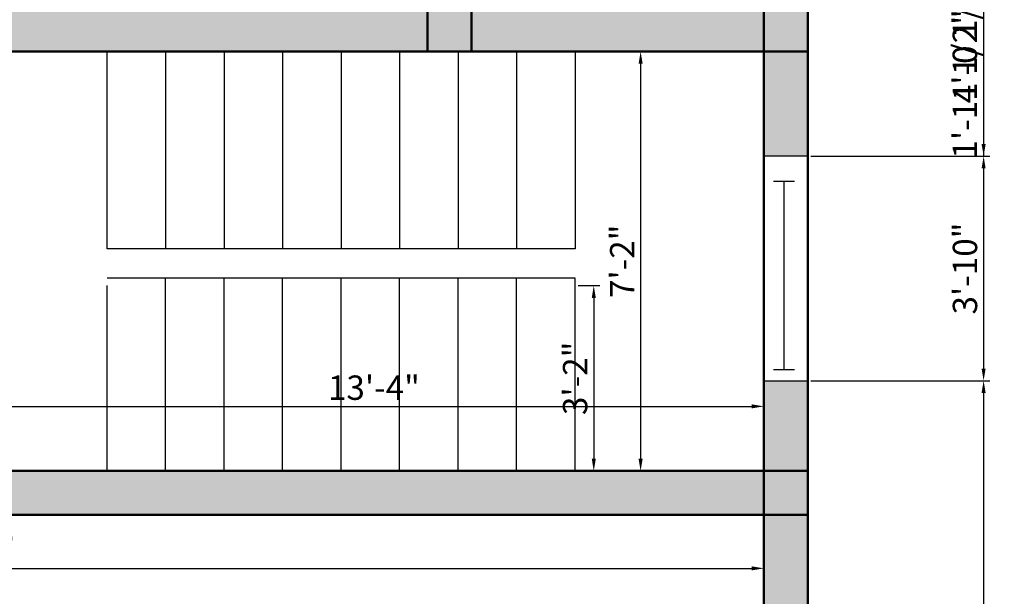
# Model space of a CAD drawing. Units: millimetres. Extents: x 2784 to 3697, y 603 to 1406.
# Tile 4 of 10: x 3013 to 3215, y 959 to 1077. Entities that reach past the tile are written whole.
import ezdxf

# ---------------------------------------------------------------- set-up
doc = ezdxf.new("R2010")
doc.units = ezdxf.units.MM
for name, color, linetype, lineweight in [('A-ANNO-DIMS', 140, 'Continuous', 18), ('A-FLOR-STRS', 200, 'Continuous', 25), ('A-GLAZ', 30, 'Continuous', 25), ('A-WALL', 2, 'Continuous', 50), ('A-WALL-PATT', 8, 'Continuous', 13)]:
    doc.layers.add(name, color=color, linetype=linetype, lineweight=lineweight)
doc.styles.get("Standard").update_dxf_attribs({"font": 'arial.ttf'})
doc.dimstyles.new('ISO-25', dxfattribs={"dimtxt": 5, "dimasz": 2.5, "dimexe": 1.25, "dimexo": 0.625, "dimtad": 1, "dimdec": 0, "dimlunit": 3, "dimtxsty": 'Standard', "dimcen": 2.5, "dimadec": 0, "dimazin": 0, "dimtfac": 1, "dimtdec": 0, "dimtmove": 0, "dimatfit": 3, "dimfxl": 1, "dimarcsym": 0})

# ---------------------------------------------------------------- blocks, each defined once
blk = doc.blocks.new('*U4')
for p, q in [((0, 4), (0, 0)), ((36, 4), (36, 0)), ((0, 2), (36, 2))]:
    blk.add_line(p, q)
blk = doc.blocks.new('*D27')
at = {"layer": 'A-ANNO-DIMS', "color": 0, "lineweight": -2, "transparency": 16777216}
for p, q in [((3005.91, 1000.77), (3005.91, 996.23)), ((3165.91, 1000.77), (3165.91, 996.23)), ((3008.41, 997.48), (3163.41, 997.48))]:
    blk.add_line(p, q, dxfattribs=at)
at = {"layer": 'A-ANNO-DIMS', "color": 0, "transparency": 16777216}
for points in [[(3008.41, 997.9), (3008.41, 997.06), (3005.91, 997.48)], [(3163.41, 997.9), (3163.41, 997.06), (3165.91, 997.48)]]:
    blk.add_solid(points, dxfattribs=at)
at = {"layer": 'Defpoints', "color": 0, "transparency": 16777216}
for p in [(3005.91, 1001.39), (3165.91, 1001.39), (3165.91, 997.48)]:
    blk.add_point(p, dxfattribs=at)
at = {"layer": 'A-ANNO-DIMS', "color": 0, "transparency": 16777216, "insert": (3085.91, 1000.66), "char_height": 5, "attachment_point": 5}
blk.add_mtext('13\'-4"', dxfattribs=at)
blk = doc.blocks.new('*D28')
at = {"layer": 'A-ANNO-DIMS', "color": 0, "lineweight": -2, "transparency": 16777216}
for p, q in [((3141.26, 1070.23), (3141.88, 1070.23)), ((3140.63, 1067.73), (3140.63, 986.73)), ((3141.26, 984.23), (3141.88, 984.23))]:
    blk.add_line(p, q, dxfattribs=at)
at = {"layer": 'A-ANNO-DIMS', "color": 0, "transparency": 16777216}
for points in [[(3140.21, 1067.73), (3141.05, 1067.73), (3140.63, 1070.23)], [(3140.21, 986.73), (3141.05, 986.73), (3140.63, 984.23)]]:
    blk.add_solid(points, dxfattribs=at)
at = {"layer": 'Defpoints', "color": 0, "transparency": 16777216}
for p in [(3140.63, 1070.23), (3140.63, 984.23), (3140.63, 984.23)]:
    blk.add_point(p, dxfattribs=at)
at = {"layer": 'A-ANNO-DIMS', "color": 0, "transparency": 16777216, "insert": (3137.5, 1027.23), "char_height": 5, "attachment_point": 5, "rotation": 90}
blk.add_mtext('7\'-2"', dxfattribs=at)
blk = doc.blocks.new('*D29')
at = {"layer": 'A-ANNO-DIMS', "color": 0, "lineweight": -2, "transparency": 16777216}
for p, q in [((3127.81, 1022.23), (3132.27, 1022.23)), ((3131.02, 1019.73), (3131.02, 986.73)), ((3127.81, 984.23), (3132.27, 984.23))]:
    blk.add_line(p, q, dxfattribs=at)
at = {"layer": 'A-ANNO-DIMS', "color": 0, "transparency": 16777216}
for points in [[(3130.61, 1019.73), (3131.44, 1019.73), (3131.02, 1022.23)], [(3130.61, 986.73), (3131.44, 986.73), (3131.02, 984.23)]]:
    blk.add_solid(points, dxfattribs=at)
at = {"layer": 'Defpoints', "color": 0, "transparency": 16777216}
for p in [(3127.18, 1022.23), (3127.18, 984.23), (3131.02, 984.23)]:
    blk.add_point(p, dxfattribs=at)
at = {"layer": 'A-ANNO-DIMS', "color": 0, "transparency": 16777216, "insert": (3127.84, 1003.23), "char_height": 5, "attachment_point": 5, "rotation": 90}
blk.add_mtext('3\'-2"', dxfattribs=at)
blk = doc.blocks.new('*D35')
at = {"layer": 'A-ANNO-DIMS', "color": 0, "lineweight": -2, "transparency": 16777216}
for p, q in [((2839.91, 959.54), (2839.91, 965.51)), ((2842.41, 964.26), (3163.41, 964.26)), ((3165.91, 959.54), (3165.91, 965.51))]:
    blk.add_line(p, q, dxfattribs=at)
at = {"layer": 'A-ANNO-DIMS', "color": 0, "transparency": 16777216}
for points in [[(2842.41, 964.68), (2842.41, 963.84), (2839.91, 964.26)], [(3163.41, 964.68), (3163.41, 963.84), (3165.91, 964.26)]]:
    blk.add_solid(points, dxfattribs=at)
at = {"layer": 'Defpoints', "color": 0, "transparency": 16777216}
for p in [(3165.91, 964.26), (2839.91, 958.92), (3165.91, 958.92)]:
    blk.add_point(p, dxfattribs=at)
at = {"layer": 'A-ANNO-DIMS', "color": 0, "transparency": 16777216, "insert": (3002.91, 967.39), "char_height": 5, "attachment_point": 5}
blk.add_mtext('27\'-2"', dxfattribs=at)
blk = doc.blocks.new('*D97')
at = {"layer": 'A-ANNO-DIMS', "color": 0, "lineweight": -2, "transparency": 16777216}
for p, q in [((3175.53, 1097.37), (3212.26, 1097.37)), ((3211.01, 1094.87), (3211.01, 1051.27)), ((3175.53, 1048.77), (3212.26, 1048.77))]:
    blk.add_line(p, q, dxfattribs=at)
at = {"layer": 'A-ANNO-DIMS', "color": 0, "transparency": 16777216}
for points in [[(3210.59, 1094.87), (3211.42, 1094.87), (3211.01, 1097.37)], [(3210.59, 1051.27), (3211.42, 1051.27), (3211.01, 1048.77)]]:
    blk.add_solid(points, dxfattribs=at)
at = {"layer": 'Defpoints', "color": 0, "transparency": 16777216}
for p in [(3174.91, 1097.37), (3174.91, 1048.77), (3211.01, 1048.77)]:
    blk.add_point(p, dxfattribs=at)
at = {"layer": 'A-ANNO-DIMS', "color": 0, "transparency": 16777216, "insert": (3207.8, 1073.07), "char_height": 5, "attachment_point": 5, "rotation": 90}
blk.add_mtext('4\'-0 1/2"', dxfattribs=at)
blk = doc.blocks.new('*D98')
at = {"layer": 'A-ANNO-DIMS', "color": 0, "lineweight": -2, "transparency": 16777216}
for p, q in [((3175.53, 1048.77), (3212.26, 1048.77)), ((3211.01, 1046.27), (3211.01, 1005.24)), ((3175.53, 1002.74), (3212.26, 1002.74))]:
    blk.add_line(p, q, dxfattribs=at)
at = {"layer": 'A-ANNO-DIMS', "color": 0, "transparency": 16777216}
for points in [[(3210.59, 1046.27), (3211.42, 1046.27), (3211.01, 1048.77)], [(3210.59, 1005.24), (3211.42, 1005.24), (3211.01, 1002.74)]]:
    blk.add_solid(points, dxfattribs=at)
at = {"layer": 'Defpoints', "color": 0, "transparency": 16777216}
for p in [(3174.91, 1048.77), (3174.91, 1002.74), (3211.01, 1002.74)]:
    blk.add_point(p, dxfattribs=at)
at = {"layer": 'A-ANNO-DIMS', "color": 0, "transparency": 16777216, "insert": (3207.83, 1025.75), "char_height": 5, "attachment_point": 5, "rotation": 90}
blk.add_mtext('3\'-10"', dxfattribs=at)
blk = doc.blocks.new('*D99')
at = {"layer": 'A-ANNO-DIMS', "color": 0, "lineweight": -2, "transparency": 16777216}
for p, q in [((3175.53, 1002.74), (3212.26, 1002.74)), ((3211.01, 1000.24), (3211.01, 646.1)), ((3175.53, 643.6), (3212.26, 643.6))]:
    blk.add_line(p, q, dxfattribs=at)
at = {"layer": 'A-ANNO-DIMS', "color": 0, "transparency": 16777216}
for points in [[(3210.59, 1000.24), (3211.42, 1000.24), (3211.01, 1002.74)], [(3210.59, 646.1), (3211.42, 646.1), (3211.01, 643.6)]]:
    blk.add_solid(points, dxfattribs=at)
at = {"layer": 'Defpoints', "color": 0, "transparency": 16777216}
for p in [(3174.91, 1002.74), (3174.91, 643.6), (3211.01, 643.6)]:
    blk.add_point(p, dxfattribs=at)
at = {"layer": 'A-ANNO-DIMS', "color": 0, "transparency": 16777216, "insert": (3207.83, 823.17), "char_height": 5, "attachment_point": 5, "rotation": 90}
blk.add_mtext('29\'-11"', dxfattribs=at)
blk = doc.blocks.new('*D107')
at = {"layer": 'A-ANNO-DIMS', "color": 0, "lineweight": -2, "transparency": 16777216}
for p, q in [((3105.04, 1104.19), (3212.26, 1104.19)), ((3211.01, 1101.69), (3211.01, 1083.41)), ((3106.53, 1080.91), (3212.26, 1080.91)), ((3211.01, 1080.91), (3211.01, 1048.8))]:
    blk.add_line(p, q, dxfattribs=at)
at = {"layer": 'A-ANNO-DIMS', "color": 0, "transparency": 16777216}
for points in [[(3210.59, 1101.69), (3211.42, 1101.69), (3211.01, 1104.19)], [(3210.59, 1083.41), (3211.42, 1083.41), (3211.01, 1080.91)]]:
    blk.add_solid(points, dxfattribs=at)
at = {"layer": 'Defpoints', "color": 0, "transparency": 16777216}
for p in [(3104.41, 1104.19), (3105.91, 1080.91), (3211.01, 1080.91)]:
    blk.add_point(p, dxfattribs=at)
at = {"layer": 'A-ANNO-DIMS', "color": 0, "transparency": 16777216, "insert": (3207.8, 1063.61), "char_height": 5, "attachment_point": 5, "rotation": 90}
blk.add_mtext('1\'-11 1/2"', dxfattribs=at)

msp = doc.modelspace()

# ---------------------------------------------------------------- hatches: boundary and pattern name
at = {"layer": 'A-WALL-PATT'}
h = msp.add_hatch(color=256, dxfattribs=at)
h.dxf.hatch_style = 1
h.paths.add_polyline_path([(2869.53, 1356.23), (2839.91, 1356.23), (2839.91, 1347.23), (2869.53, 1347.23)])
h.paths.add_polyline_path([(2839.91, 1356.23), (2830.91, 1356.23), (2830.91, 1347.23), (2839.91, 1347.23)])
h.paths.add_polyline_path([(2839.91, 1347.23), (2830.91, 1347.23), (2830.91, 1314.23), (2839.91, 1314.23)])
h.paths.add_polyline_path([(2839.91, 1268.19), (2830.91, 1268.19), (2830.91, 1222.23), (2839.91, 1222.23)])
h.paths.add_polyline_path([(2839.91, 1222.23), (2830.91, 1222.23), (2830.91, 1213.23), (2839.91, 1213.23)])
h.paths.add_polyline_path([(2962.91, 1222.23), (2839.91, 1222.23), (2839.91, 1213.23), (2962.91, 1213.23)])
h.paths.add_polyline_path([(2971.91, 1222.23), (2962.91, 1222.23), (2962.91, 1213.23), (2971.91, 1213.23)])
h.paths.add_polyline_path([(2971.91, 1263.23), (2962.91, 1263.23), (2962.91, 1254.23), (2971.91, 1254.23)])
h.paths.add_polyline_path([(2971.91, 1347.23), (2962.91, 1347.23), (2962.91, 1263.23), (2971.91, 1263.23)])
h.paths.add_polyline_path([(2971.91, 1356.23), (2962.91, 1356.23), (2962.91, 1347.23), (2971.91, 1347.23)])
h.paths.add_polyline_path([(2962.91, 1356.23), (2913.7, 1356.23), (2913.7, 1347.23), (2962.91, 1347.23)])
h.paths.add_polyline_path([(2982.62, 1356.23), (2971.91, 1356.23), (2971.91, 1347.23), (2982.62, 1347.23)])
h.paths.add_polyline_path([(3019.91, 1356.23), (3004.44, 1356.23), (3004.44, 1347.23), (3019.91, 1347.23)])
h.paths.add_polyline_path([(3028.91, 1356.23), (3019.91, 1356.23), (3019.91, 1347.23), (3028.91, 1347.23)])
h.paths.add_polyline_path([(3028.91, 1347.23), (3019.91, 1347.23), (3019.91, 1287.35, -0.06506), (3026.12, 1288.16), (3028.91, 1288.16)])
h.paths.add_polyline_path([(3019.91, 1263.23), (2971.91, 1263.23), (2971.91, 1254.23), (3019.91, 1254.23)])
h.paths.add_polyline_path([(3028.91, 1263.23), (3019.91, 1263.23), (3019.91, 1254.23), (3028.91, 1254.23)])
h.paths.add_polyline_path([(3028.91, 1254.23), (3019.91, 1254.23), (3019.91, 1222.23), (3028.91, 1222.23)])
h.paths.add_polyline_path([(3028.91, 1222.23), (3019.91, 1222.23), (3019.91, 1213.23), (3028.91, 1213.23)])
h.paths.add_polyline_path([(3165.91, 1222.23), (3060.65, 1222.23, -0.056956), (3061.45, 1215.23), (3061.45, 1213.23), (3165.91, 1213.23)])
h.paths.add_polyline_path([(3080.34, 1356.23), (3028.91, 1356.23), (3028.91, 1347.23), (3080.34, 1347.23)])
h.paths.add_polyline_path([(3174.91, 1347.23), (3165.91, 1347.23), (3165.91, 1311.28), (3174.91, 1311.28)])
h.paths.add_polyline_path([(3174.91, 1356.23), (3165.91, 1356.23), (3165.91, 1347.23), (3174.91, 1347.23)])
h.paths.add_polyline_path([(3165.91, 1356.23), (3123.1, 1356.23), (3123.1, 1347.23), (3165.91, 1347.23)])
h.paths.add_polyline_path([(3174.91, 1266.65), (3165.91, 1266.65), (3165.91, 1222.23), (3174.91, 1222.23)])
h.paths.add_polyline_path([(3174.91, 1222.23), (3165.91, 1222.23), (3165.91, 1213.23), (3174.91, 1213.23)])
h.paths.add_polyline_path([(3174.91, 1213.23), (3165.91, 1213.23), (3165.91, 1194.83), (3174.91, 1194.83)])
h.paths.add_polyline_path([(3105.91, 1182.92, -0.096276), (3096.91, 1180.92), (3096.91, 1148.23), (3105.91, 1148.23)])
h.paths.add_polyline_path([(3105.91, 1213.23), (3096.91, 1213.23), (3096.91, 1205.07), (3105.91, 1205.07)])
h.paths.add_polyline_path([(2971.91, 1213.23), (2962.91, 1213.23), (2962.91, 1161.09), (2971.91, 1161.09)])
h.paths.add_polyline_path([(2839.91, 1213.23), (2830.91, 1213.23), (2830.91, 1157.46), (2839.91, 1157.46)])
h.paths.add_polyline_path([(2839.91, 1108.88), (2830.91, 1108.88), (2830.91, 1042.23), (2839.91, 1042.23)])
h.paths.add_polyline_path([(2839.91, 1042.23), (2830.91, 1042.23), (2830.91, 1033.23), (2839.91, 1033.23)])
h.paths.add_polyline_path([(2881.91, 1042.23), (2839.91, 1042.23), (2839.91, 1033.23), (2881.91, 1033.23)])
h.paths.add_polyline_path([(2996.91, 1042.23), (2890.91, 1042.23), (2890.91, 1033.23), (2996.91, 1033.23)])
h.paths.add_polyline_path([(2890.91, 1042.23), (2881.91, 1042.23), (2881.91, 1033.23), (2890.91, 1033.23)])
h.paths.add_polyline_path([(2890.91, 1033.23), (2881.91, 1033.23), (2881.91, 984.23), (2890.91, 984.23)])
h.paths.add_polyline_path([(2839.91, 1033.23), (2830.91, 1033.23), (2830.91, 984.23), (2839.91, 984.23)])
h.paths.add_polyline_path([(2839.91, 984.23), (2830.91, 984.23), (2830.91, 975.23), (2839.91, 975.23)])
h.paths.add_polyline_path([(2881.91, 984.23), (2854.14, 984.23, -0.154991), (2857.05, 975.23), (2881.91, 975.23)])
h.paths.add_polyline_path([(2890.91, 984.23), (2881.91, 984.23), (2881.91, 975.23), (2890.91, 975.23)])
h.paths.add_polyline_path([(2900.85, 984.23), (2890.91, 984.23), (2890.91, 975.23), (2900.85, 975.23), (2900.85, 975.78)])
h.paths.add_polyline_path([(2996.91, 984.23), (2923.49, 984.23, -0.089525), (2925.01, 975.78), (2925.01, 975.23), (2996.91, 975.23)])
h.paths.add_polyline_path([(3165.91, 984.23), (3005.91, 984.23), (3005.91, 975.23), (3165.91, 975.23)])
h.paths.add_polyline_path([(3005.91, 1033.23), (2996.91, 1033.23), (2996.91, 984.23), (3005.91, 984.23)])
h.paths.add_polyline_path([(3005.91, 984.23), (2996.91, 984.23), (2996.91, 975.23), (3005.91, 975.23)])
h.paths.add_polyline_path([(3005.91, 1042.23), (2996.91, 1042.23), (2996.91, 1033.23), (3005.91, 1033.23)])
h.paths.add_polyline_path([(3096.91, 1079.23), (2971.91, 1079.23), (2971.91, 1070.23), (3096.91, 1070.23)])
h.paths.add_polyline_path([(2971.91, 1079.23), (2962.91, 1079.23), (2962.91, 1070.23), (2971.91, 1070.23)])
h.paths.add_polyline_path([(2971.91, 1070.23), (2962.91, 1070.23), (2962.91, 1060.28, -0.115005), (2971.91, 1066.55)])
h.paths.add_polyline_path([(2971.91, 1105.54), (2962.91, 1105.54), (2962.91, 1079.23), (2971.91, 1079.23)])
h.paths.add_polyline_path([(3165.91, 1079.23), (3105.91, 1079.23), (3105.91, 1070.23), (3165.91, 1070.23)])
h.paths.add_polyline_path([(3105.91, 1079.23), (3096.91, 1079.23), (3096.91, 1070.23), (3105.91, 1070.23)])
h.paths.add_polyline_path([(3105.91, 1148.23), (3096.91, 1148.23), (3096.91, 1139.23), (3105.91, 1139.23)])
h.paths.add_polyline_path([(3105.91, 1139.23), (3096.91, 1139.23), (3096.91, 1104.7), (3098.08, 1104.75, -0.08216), (3105.91, 1103.81)])
h.paths.add_polyline_path([(3165.91, 1148.23), (3105.91, 1148.23), (3105.91, 1139.23), (3165.91, 1139.23)])
h.paths.add_polyline_path([(3174.91, 1148.23), (3165.91, 1148.23), (3165.91, 1139.23), (3174.91, 1139.23)])
h.paths.add_polyline_path([(3174.91, 1139.23), (3165.91, 1139.23), (3165.91, 1123.86), (3174.91, 1123.86)])
h.paths.add_polyline_path([(3174.91, 1097.37), (3165.91, 1097.37), (3165.91, 1079.23), (3174.91, 1079.23)])
h.paths.add_polyline_path([(3174.91, 1079.23), (3165.91, 1079.23), (3165.91, 1070.23), (3174.91, 1070.23)])
h.paths.add_polyline_path([(3174.91, 1070.23), (3165.91, 1070.23), (3165.91, 1048.77), (3174.91, 1048.77)])
h.paths.add_polyline_path([(3174.91, 1002.74), (3165.91, 1002.74), (3165.91, 984.23), (3174.91, 984.23)])
h.paths.add_polyline_path([(3174.91, 984.23), (3165.91, 984.23), (3165.91, 975.23), (3174.91, 975.23)])
h.paths.add_polyline_path([(3174.91, 975.23), (3165.91, 975.23), (3165.91, 725.23), (3174.91, 725.23)])
h.paths.add_polyline_path([(2839.91, 975.23), (2830.91, 975.23), (2830.91, 725.23), (2839.91, 725.23)])
h.paths.add_polyline_path([(3165.91, 725.23), (2839.91, 725.23), (2839.91, 716.23), (3165.91, 716.23)])
h.paths.add_polyline_path([(3174.91, 725.23), (3165.91, 725.23), (3165.91, 716.23), (3174.91, 716.23)])
h.paths.add_polyline_path([(2839.91, 725.23), (2830.91, 725.23), (2830.91, 716.23), (2839.91, 716.23)])

# ---------------------------------------------------------------- linework, layer by layer
at = {"layer": 'A-FLOR-STRS'}
for p, q in [((3031.18, 1029.78), (3031.18, 1070.23)), ((3043.18, 1070.23), (3043.18, 1032.34)), ((3043.18, 1070.23), (3043.18, 1029.78)), ((3055.18, 1070.23), (3055.18, 1032.34)), ((3055.18, 1070.23), (3055.18, 1029.78)), ((3067.18, 1070.23), (3067.18, 1032.34)), ((3067.18, 1070.23), (3067.18, 1029.78)), ((3079.18, 1070.23), (3079.18, 1032.34)), ((3079.18, 1070.23), (3079.18, 1029.78)), ((3091.18, 1070.23), (3091.18, 1032.34)), ((3091.18, 1070.23), (3091.18, 1029.78)), ((3103.18, 1070.23), (3103.18, 1032.34)), ((3103.18, 1070.23), (3103.18, 1029.78)), ((3115.18, 1070.23), (3115.18, 1032.34)), ((3115.18, 1070.23), (3115.18, 1029.78)), ((3127.18, 1070.23), (3127.18, 1032.34)), ((3127.18, 1070.23), (3127.18, 1029.78)), ((3127.18, 1029.78), (3031.18, 1029.78)), ((3127.18, 1023.8), (3031.18, 1023.8)), ((3043.18, 984.23), (3043.18, 1023.8)), ((3055.18, 984.23), (3055.18, 1023.8)), ((3067.18, 984.23), (3067.18, 1023.8)), ((3079.18, 984.23), (3079.18, 1023.8)), ((3091.18, 984.23), (3091.18, 1023.8)), ((3103.18, 984.23), (3103.18, 1023.8)), ((3115.18, 984.23), (3115.18, 1023.8)), ((3127.18, 984.23), (3127.18, 1023.8)), ((3031.18, 984.23), (3031.18, 1022.23)), ((3043.18, 984.23), (3043.18, 1022.23)), ((3055.18, 984.23), (3055.18, 1022.23)), ((3067.18, 984.23), (3067.18, 1022.23)), ((3079.18, 984.23), (3079.18, 1022.23)), ((3091.18, 984.23), (3091.18, 1022.23)), ((3103.18, 984.23), (3103.18, 1022.23)), ((3115.18, 984.23), (3115.18, 1022.23)), ((3127.18, 984.23), (3127.18, 1022.23))]:
    msp.add_line(p, q, dxfattribs=at)
at = {"layer": 'A-GLAZ'}
for p, q in [((3174.91, 1048.77), (3165.91, 1048.77)), ((3165.91, 1002.74), (3174.91, 1002.74))]:
    msp.add_line(p, q, dxfattribs=at)
at = {"layer": 'A-WALL'}
for p, q in [((3165.91, 1213.23), (3165.91, 643.6)), ((3174.91, 1213.23), (3174.91, 643.6)), ((3105.91, 1080.91), (3105.91, 1070.23)), ((3096.91, 1080.52), (3096.91, 1070.23)), ((2962.91, 1070.23), (3174.91, 1070.23)), ((2923.49, 984.23), (3174.91, 984.23)), ((2925.01, 975.23), (3174.91, 975.23))]:
    msp.add_line(p, q, dxfattribs=at)

# ---------------------------------------------------------------- block references
at = {"layer": 'A-GLAZ', "xscale": 1.074021802203067, "yscale": 1.074021802203067, "zscale": 1.074021802203067, "rotation": 270}
msp.add_blockref('*U4', (3167.9, 1043.6), dxfattribs=at)

# ---------------------------------------------------------------- dimensions: what is measured, and where the dimension line sits
at = {"layer": 'A-ANNO-DIMS'}
for base, p1, p2, override, picture, middle in [((3211.01, 1080.91), (3104.41, 1104.19), (3105.91, 1080.91), {"dimdec": 1, "dimlfac": 1, "dimrnd": 0, "dimzin": 1, "dimdsep": 46, "dimlunit": 4, "dimfrac": 2}, '*D107', (3207.8, 1063.61)), ((3211.01, 1048.77), (3174.91, 1097.37), (3174.91, 1048.77), {"dimdec": 1, "dimlfac": 1, "dimrnd": 0, "dimzin": 1, "dimdsep": 46, "dimlunit": 4, "dimfrac": 2}, '*D97', (3207.8, 1073.07)), ((3140.63, 984.23), (3140.63, 1070.23), (3140.63, 984.23), {"dimclrd": 0, "dimclre": 0, "dimclrt": 0}, '*D28', (3137.5, 1027.23)), ((3211.01, 1002.74), (3174.91, 1048.77), (3174.91, 1002.74), {"dimdec": 1, "dimlfac": 1, "dimrnd": 0, "dimzin": 1, "dimdsep": 46, "dimlunit": 4, "dimfrac": 2}, '*D98', (3207.83, 1025.75)), ((3131.02, 984.23), (3127.18, 1022.23), (3127.18, 984.23), {"dimclrd": 0, "dimclre": 0, "dimclrt": 0}, '*D29', (3127.84, 1003.23)), ((3211.01, 643.6), (3174.91, 1002.74), (3174.91, 643.6), {"dimdec": 1, "dimlfac": 1, "dimrnd": 0, "dimzin": 1, "dimdsep": 46, "dimlunit": 4, "dimfrac": 2}, '*D99', (3207.83, 823.17))]:
    dim = msp.add_linear_dim(base=base, p1=p1, p2=p2, angle=90, dimstyle='ISO-25', override=override, dxfattribs=at)
    dim.commit()
    dim.dimension.update_dxf_attribs({"geometry": picture, "text_midpoint": middle})
for base, p1, p2, picture, middle in [((3165.91, 997.48), (3005.91, 1001.39), (3165.91, 1001.39), '*D27', (3085.91, 1000.66)), ((3165.91, 964.26), (2839.91, 958.92), (3165.91, 958.92), '*D35', (3002.91, 967.39))]:
    dim = msp.add_linear_dim(base=base, p1=p1, p2=p2, dimstyle='ISO-25', override={"dimclrd": 0, "dimclre": 0, "dimclrt": 0}, dxfattribs=at)
    dim.commit()
    dim.dimension.update_dxf_attribs({"geometry": picture, "text_midpoint": middle})

doc.saveas('drawing.dxf')
